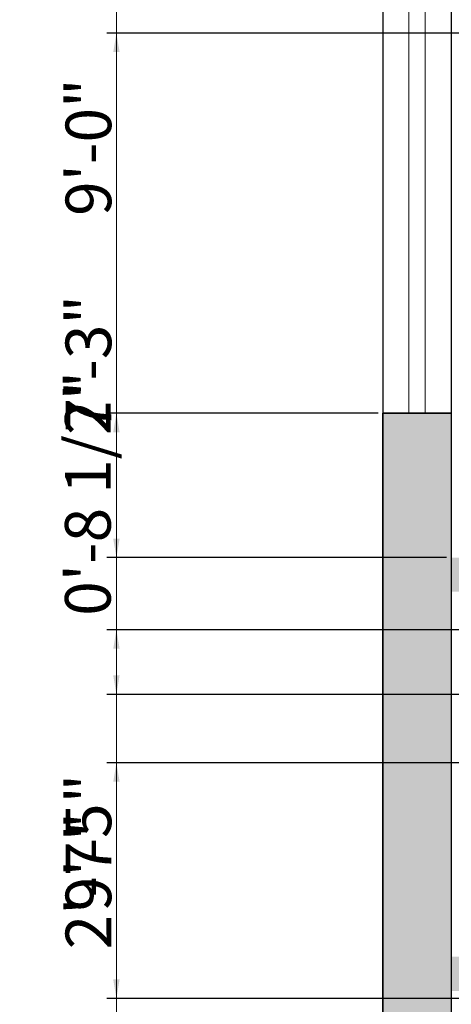
# Model space of a CAD drawing. Units: inches. Extents: x 2696 to 3240, y 1564 to 2310.
# Tile 14 of 76: x 2698 to 2755, y 1852 to 1982. Entities that reach past the tile are written whole.
import ezdxf

# ---------------------------------------------------------------- set-up
doc = ezdxf.new("R2010")
doc.units = ezdxf.units.IN
for name, color, linetype, lineweight in [('A-ANNO-DIMS', 3, 'Continuous', 18), ('A-WALL', 7, 'Continuous', 35), ('A-WALL-PATT', 9, 'Continuous', 13), ('WINDOW', 2, 'Continuous', 18)]:
    doc.layers.add(name, color=color, linetype=linetype, lineweight=lineweight)
doc.styles.add('TIMES NEW', font='times.ttf')
doc.dimstyles.new('Siddhuu', dxfattribs={"dimtxt": 6, "dimasz": 2.5, "dimexe": 1.25, "dimexo": 0.625, "dimtad": 1, "dimdec": 1, "dimlunit": 4, "dimtxsty": 'TIMES NEW', "dimcen": 2.5, "dimclrd": 256, "dimclre": 1, "dimclrt": 7, "dimadec": 0, "dimazin": 0, "dimtfac": 1, "dimtdec": 1, "dimtmove": 0, "dimatfit": 3, "dimfxl": 1, "dimtolj": 1, "dimlwd": -1, "dimarcsym": 0})

# ---------------------------------------------------------------- blocks, each defined once
blk = doc.blocks.new('WD_WIN4')
for p, q in [((-0.5, 0.5), (0.5, 0.5)), ((-0.5, 0.12), (0.5, 0.12)), ((-0.5, -0.12), (0.5, -0.12)), ((-0.5, -0.5), (0.5, -0.5))]:
    blk.add_line(p, q)
blk = doc.blocks.new('*D55')
at = {"layer": 'A-ANNO-DIMS', "color": 1, "lineweight": -2, "transparency": 16777216}
for p, q in [((3189.99, 1980.2), (2709.36, 1980.2)), ((3189.99, 1893.2), (2709.36, 1893.2))]:
    blk.add_line(p, q, dxfattribs=at)
at = {"layer": 'A-ANNO-DIMS', "transparency": 16777216}
blk.add_line((2710.61, 1895.7), (2710.61, 1977.7), dxfattribs=at)
for points in [[(2710.19, 1977.7), (2711.03, 1977.7), (2710.61, 1980.2)], [(2710.19, 1895.7), (2711.03, 1895.7), (2710.61, 1893.2)]]:
    blk.add_solid(points, dxfattribs=at)
at = {"layer": 'Defpoints', "color": 0, "transparency": 16777216}
for p in [(2710.61, 1980.2), (3190.61, 1980.2), (3190.61, 1893.2)]:
    blk.add_point(p, dxfattribs=at)
at = {"layer": 'A-ANNO-DIMS', "color": 7, "transparency": 16777216, "insert": (2706.93, 1936.7), "char_height": 6, "attachment_point": 5, "rotation": 90, "style": 'TIMES NEW'}
blk.add_mtext('\\A1;7\'-3"', dxfattribs=at)
blk = doc.blocks.new('*D57')
at = {"layer": 'A-ANNO-DIMS', "color": 1, "lineweight": -2, "transparency": 16777216}
for p, q in [((2754.61, 2018.58), (2754.61, 1568.95)), ((2956.71, 2018.58), (2956.71, 1568.95))]:
    blk.add_line(p, q, dxfattribs=at)
at = {"layer": 'A-ANNO-DIMS', "transparency": 16777216}
blk.add_line((2757.11, 1570.2), (2954.21, 1570.2), dxfattribs=at)
for points in [[(2757.11, 1570.62), (2757.11, 1569.78), (2754.61, 1570.2)], [(2954.21, 1570.62), (2954.21, 1569.78), (2956.71, 1570.2)]]:
    blk.add_solid(points, dxfattribs=at)
at = {"layer": 'Defpoints', "color": 0, "transparency": 16777216}
for p in [(2754.61, 2019.2), (2956.71, 2019.2), (2956.71, 1570.2)]:
    blk.add_point(p, dxfattribs=at)
at = {"layer": 'A-ANNO-DIMS', "color": 7, "transparency": 16777216, "insert": (2855.66, 1573.88), "char_height": 6, "attachment_point": 5, "style": 'TIMES NEW'}
blk.add_mtext('\\A1;16\'-10"', dxfattribs=at)
blk = doc.blocks.new('*D58')
at = {"layer": 'A-ANNO-DIMS', "color": 1, "lineweight": -2, "transparency": 16777216}
for p, q in [((2753.99, 2019.2), (2709.36, 2019.2)), ((2753.99, 1911.2), (2709.36, 1911.2))]:
    blk.add_line(p, q, dxfattribs=at)
at = {"layer": 'A-ANNO-DIMS', "transparency": 16777216}
blk.add_line((2710.61, 1913.7), (2710.61, 2016.7), dxfattribs=at)
for points in [[(2710.19, 2016.7), (2711.03, 2016.7), (2710.61, 2019.2)], [(2710.19, 1913.7), (2711.03, 1913.7), (2710.61, 1911.2)]]:
    blk.add_solid(points, dxfattribs=at)
at = {"layer": 'Defpoints', "color": 0, "transparency": 16777216}
for p in [(2710.61, 2019.2), (2754.61, 2019.2), (2754.61, 1911.2)]:
    blk.add_point(p, dxfattribs=at)
at = {"layer": 'A-ANNO-DIMS', "color": 7, "transparency": 16777216, "insert": (2706.93, 1965.2), "char_height": 6, "attachment_point": 5, "rotation": 90, "style": 'TIMES NEW'}
blk.add_mtext('\\A1;9\'-0"', dxfattribs=at)
blk = doc.blocks.new('*D68')
at = {"layer": 'A-ANNO-DIMS', "color": 1, "lineweight": -2, "transparency": 16777216}
for p, q in [((2745.61, 2261.58), (2745.61, 1568.95)), ((2782.83, 2261.58), (2782.83, 1568.95))]:
    blk.add_line(p, q, dxfattribs=at)
at = {"layer": 'A-ANNO-DIMS', "transparency": 16777216}
blk.add_line((2748.11, 1570.2), (2780.33, 1570.2), dxfattribs=at)
for points in [[(2748.11, 1570.62), (2748.11, 1569.78), (2745.61, 1570.2)], [(2780.33, 1570.62), (2780.33, 1569.78), (2782.83, 1570.2)]]:
    blk.add_solid(points, dxfattribs=at)
at = {"layer": 'Defpoints', "color": 0, "transparency": 16777216}
for p in [(2745.61, 2262.2), (2782.83, 2262.2), (2782.83, 1570.2)]:
    blk.add_point(p, dxfattribs=at)
at = {"layer": 'A-ANNO-DIMS', "color": 7, "transparency": 16777216, "insert": (2764.22, 1573.88), "char_height": 6, "attachment_point": 5, "style": 'TIMES NEW'}
blk.add_mtext('\\A1;3\'-1"', dxfattribs=at)
blk = doc.blocks.new('*D73')
at = {"layer": 'A-ANNO-DIMS', "color": 1, "lineweight": -2, "transparency": 16777216}
for p, q in [((2744.99, 1930.2), (2709.36, 1930.2)), ((2744.99, 1817.2), (2709.36, 1817.2))]:
    blk.add_line(p, q, dxfattribs=at)
at = {"layer": 'A-ANNO-DIMS', "transparency": 16777216}
blk.add_line((2710.61, 1927.7), (2710.61, 1819.7), dxfattribs=at)
for points in [[(2710.19, 1927.7), (2711.03, 1927.7), (2710.61, 1930.2)], [(2710.19, 1819.7), (2711.03, 1819.7), (2710.61, 1817.2)]]:
    blk.add_solid(points, dxfattribs=at)
at = {"layer": 'Defpoints', "color": 0, "transparency": 16777216}
for p in [(2745.61, 1930.2), (2710.61, 1817.2), (2745.61, 1817.2)]:
    blk.add_point(p, dxfattribs=at)
at = {"layer": 'A-ANNO-DIMS', "color": 7, "transparency": 16777216, "insert": (2706.93, 1873.7), "char_height": 6, "attachment_point": 5, "rotation": 90, "style": 'TIMES NEW'}
blk.add_mtext('\\A1;9\'-5"', dxfattribs=at)
blk = doc.blocks.new('*D78')
at = {"layer": 'A-ANNO-DIMS', "transparency": 16777216}
for p, q in [((2710.61, 1901.7), (2710.61, 1935.1)), ((2710.61, 1895.7), (2710.61, 1899.2))]:
    blk.add_line(p, q, dxfattribs=at)
at = {"layer": 'A-ANNO-DIMS', "color": 1, "lineweight": -2, "transparency": 16777216}
for p, q in [((3189.99, 1901.7), (2709.36, 1901.7)), ((3189.99, 1893.2), (2709.36, 1893.2))]:
    blk.add_line(p, q, dxfattribs=at)
at = {"layer": 'A-ANNO-DIMS', "transparency": 16777216}
for points in [[(2710.19, 1899.2), (2711.03, 1899.2), (2710.61, 1901.7)], [(2710.19, 1895.7), (2711.03, 1895.7), (2710.61, 1893.2)]]:
    blk.add_solid(points, dxfattribs=at)
at = {"layer": 'Defpoints', "color": 0, "transparency": 16777216}
for p in [(2710.61, 1901.7), (3190.61, 1901.7), (3190.61, 1893.2)]:
    blk.add_point(p, dxfattribs=at)
at = {"layer": 'A-ANNO-DIMS', "color": 7, "transparency": 16777216, "insert": (2706.85, 1919.65), "char_height": 6, "attachment_point": 5, "rotation": 90, "style": 'TIMES NEW'}
blk.add_mtext('\\A1;0\'-8 1/2"', dxfattribs=at)
blk = doc.blocks.new('*D79')
at = {"layer": 'A-ANNO-DIMS', "color": 1, "lineweight": -2, "transparency": 16777216}
for p, q in [((3189.99, 1884.2), (2709.36, 1884.2)), ((3189.99, 1853.2), (2709.36, 1853.2))]:
    blk.add_line(p, q, dxfattribs=at)
at = {"layer": 'A-ANNO-DIMS', "transparency": 16777216}
blk.add_line((2710.61, 1881.7), (2710.61, 1855.7), dxfattribs=at)
for points in [[(2710.19, 1881.7), (2711.03, 1881.7), (2710.61, 1884.2)], [(2710.19, 1855.7), (2711.03, 1855.7), (2710.61, 1853.2)]]:
    blk.add_solid(points, dxfattribs=at)
at = {"layer": 'Defpoints', "color": 0, "transparency": 16777216}
for p in [(3190.61, 1884.2), (2710.61, 1853.2), (3190.61, 1853.2)]:
    blk.add_point(p, dxfattribs=at)
at = {"layer": 'A-ANNO-DIMS', "color": 7, "transparency": 16777216, "insert": (2706.93, 1868.7), "char_height": 6, "attachment_point": 5, "rotation": 90, "style": 'TIMES NEW'}
blk.add_mtext('\\A1;2\'-7"', dxfattribs=at)

msp = doc.modelspace()

# ---------------------------------------------------------------- hatches: boundary and pattern name
at = {"layer": 'A-WALL-PATT', "transparency": 33554556}
h = msp.add_hatch(color=256, dxfattribs=at)
h.dxf.hatch_style = 1
h.paths.add_polyline_path([(2879.11, 2253.2), (2905.91, 2253.2), (2905.91, 2262.2), (2841.89, 2262.2), (2841.89, 2253.2), (2870.11, 2253.2), (2870.11, 2176.6), (2965.71, 2176.6), (2965.71, 2206.7), (2973.58, 2206.7), (2973.58, 2215.7), (2965.71, 2215.7), (2965.71, 2262.2), (2929.91, 2262.2), (2929.91, 2253.2), (2956.71, 2253.2), (2956.71, 2185.6), (2879.11, 2185.6)])
h.paths.add_polyline_path([(2782.83, 2262.2), (2745.61, 2262.2), (2745.61, 2228.73), (2754.61, 2228.73), (2754.61, 2253.2), (2782.83, 2253.2)])
h.paths.add_polyline_path([(2754.61, 2136.2), (2965.71, 2136.2), (2965.71, 2145.2), (2879.11, 2145.2), (2879.11, 2147.07), (2877.34, 2147.07), (2870.11, 2147.07), (2870.11, 2145.2), (2754.61, 2145.2), (2754.61, 2169.67), (2745.61, 2169.67), (2745.61, 2000.2), (2754.61, 2000.2), (2754.61, 2019.2), (2849.08, 2019.2), (2849.08, 2023.7), (2841.21, 2023.7), (2841.21, 2051.83), (2836.71, 2051.83), (2836.71, 2023.7), (2754.61, 2023.7), (2754.61, 2091.2), (2836.71, 2091.2), (2836.71, 2087.83), (2841.21, 2087.83), (2841.21, 2095.7), (2754.61, 2095.7)])
h.paths.add_polyline_path([(2965.71, 2136.2), (2956.71, 2136.2), (2956.71, 2023.7), (2885.08, 2023.7), (2885.08, 2019.2), (2956.71, 2019.2), (2956.71, 1950.58), (2965.71, 1950.58), (2965.71, 1980.2), (2973.58, 1980.2), (2973.58, 1989.2), (2965.71, 1989.2)])
h.paths.add_polyline_path([(2754.61, 1906.7), (2880.21, 1906.7), (2884.71, 1906.7), (2956.71, 1906.7), (2956.71, 1792.7), (2944.71, 1792.7), (2944.71, 1783.7), (2956.71, 1783.7), (2956.71, 1740.2), (2884.71, 1740.2), (2884.71, 1783.7), (2896.71, 1783.7), (2896.71, 1792.7), (2884.71, 1792.7), (2884.71, 1846.7), (2880.21, 1846.7), (2880.21, 1740.2), (2754.61, 1740.2), (2754.61, 1777.2), (2745.61, 1777.2), (2745.61, 1692.7), (2754.61, 1692.7), (2754.61, 1731.2), (2956.71, 1731.2), (2956.71, 1723.33), (2965.71, 1723.33), (2965.71, 1884.2), (2973.58, 1884.2), (2973.58, 1893.2), (2965.71, 1893.2), (2965.71, 1914.58), (2956.71, 1914.58), (2956.71, 1911.2), (2754.61, 1911.2), (2754.61, 1930.2), (2745.61, 1930.2), (2745.61, 1817.2), (2754.61, 1817.2), (2754.61, 1854.2), (2826.61, 1854.2), (2826.61, 1868.83), (2822.11, 1868.83), (2822.11, 1858.7), (2754.61, 1858.7)])
h.paths.add_polyline_path([(2965.71, 1656.2), (3008.24, 1656.2), (3008.24, 1665.2), (2965.71, 1665.2), (2965.71, 1693.33), (2956.71, 1693.33), (2956.71, 1686.2), (2934.58, 1686.2), (2934.58, 1681.7), (2956.71, 1681.7), (2956.71, 1614.2), (2896.71, 1614.2), (2896.71, 1681.7), (2904.58, 1681.7), (2904.58, 1686.2), (2892.21, 1686.2), (2892.21, 1614.2), (2858.41, 1614.2), (2858.41, 1605.2), (2965.71, 1605.2)])
h.paths.add_polyline_path([(2788.41, 1614.2), (2754.61, 1614.2), (2754.61, 1652.7), (2745.61, 1652.7), (2745.61, 1605.2), (2788.41, 1605.2)])
h.paths.add_polyline_path([(3199.61, 1633.05), (3190.61, 1633.05), (3190.61, 1614.2), (3082.61, 1614.2), (3082.61, 1665.2), (3070.24, 1665.2), (3070.24, 1656.2), (3078.11, 1656.2), (3078.11, 1605.2), (3199.61, 1605.2)])
h.paths.add_polyline_path([(3199.61, 1702.05), (3190.61, 1702.05), (3190.61, 1699.7), (3106.61, 1699.7), (3106.61, 1747.7), (3190.61, 1747.7), (3190.61, 1752.2), (3082.61, 1752.2), (3082.61, 1760.08), (3078.11, 1760.08), (3078.11, 1747.7), (3102.11, 1747.7), (3102.11, 1699.7), (3078.11, 1699.7), (3078.11, 1695.2), (3190.61, 1695.2), (3190.61, 1676.35), (3199.61, 1676.35)])
h.paths.add_polyline_path([(3199.61, 1783.2), (3190.61, 1783.2), (3190.61, 1745.35), (3199.61, 1745.35)])
h.paths.add_polyline_path([(3082.61, 1884.2), (3190.61, 1884.2), (3190.61, 1853.2), (3199.61, 1853.2), (3199.61, 1901.7), (3190.61, 1901.7), (3190.61, 1893.2), (3005.58, 1893.2), (3005.58, 1891.28), (3005.58, 1884.2), (3078.11, 1884.2), (3078.11, 1792.08), (3082.61, 1792.08)])
h.paths.add_polyline_path([(3199.61, 1994.7), (3190.61, 1994.7), (3190.61, 1989.2), (3073.71, 1989.2), (3073.71, 2034.2), (3069.21, 2034.2), (3069.21, 1989.2), (3005.58, 1989.2), (3005.58, 1980.2), (3190.61, 1980.2), (3190.61, 1971.7), (3199.61, 1971.7)])
h.paths.add_polyline_path([(3199.61, 2155.2), (3190.61, 2155.2), (3190.61, 2064.7), (3199.61, 2064.7)])
h.paths.add_polyline_path([(3190.61, 2074.7), (3106.61, 2074.7), (3106.61, 2122.7), (3190.61, 2122.7), (3190.61, 2127.2), (3082.71, 2127.2), (3082.71, 2135.08), (3073.71, 2135.08), (3073.71, 2122.7), (3102.11, 2122.7), (3102.11, 2074.7), (3069.21, 2074.7), (3069.21, 2070.2), (3190.61, 2070.2)])
h.paths.add_polyline_path([(3082.71, 2253.2), (3190.61, 2253.2), (3190.61, 2225.2), (3199.61, 2225.2), (3199.61, 2262.2), (3073.71, 2262.2), (3073.71, 2215.7), (3035.58, 2215.7), (3035.58, 2206.7), (3073.71, 2206.7), (3073.71, 2171.08), (3082.71, 2171.08)])

# ---------------------------------------------------------------- linework, layer by layer
at = {"layer": 'A-WALL'}
for p in [(2745.61, 1817.2), (2754.61, 1930.2)]:
    msp.add_line(p, (2745.61, 1930.2), dxfattribs=at)

# ---------------------------------------------------------------- block references
at = {"layer": 'WINDOW', "xscale": 70, "yscale": 8.999999999999545, "zscale": 70, "rotation": 270}
msp.add_blockref('WD_WIN4', (2750.11, 1965.2), dxfattribs=at)

# ---------------------------------------------------------------- dimensions: what is measured, and where the dimension line sits
at = {"layer": 'A-ANNO-DIMS'}
for base, p1, p2, picture, middle in [((2782.83, 1570.2), (2745.61, 2262.2), (2782.83, 2262.2), '*D68', (2764.22, 1573.88)), ((2956.71, 1570.2), (2754.61, 2019.2), (2956.71, 2019.2), '*D57', (2855.66, 1573.88))]:
    dim = msp.add_linear_dim(base=base, p1=p1, p2=p2, dimstyle='Siddhuu', override={"dimdec": 1, "dimlfac": 1, "dimrnd": 0, "dimzin": 1, "dimdsep": 46, "dimlunit": 4, "dimfrac": 2}, dxfattribs=at)
    dim.commit()
    dim.dimension.update_dxf_attribs({"geometry": picture, "text_midpoint": middle})
for base, p1, p2, picture, middle in [((2710.61, 2019.2), (2754.61, 1911.2), (2754.61, 2019.2), '*D58', (2706.93, 1965.2)), ((2710.61, 1980.2), (3190.61, 1893.2), (3190.61, 1980.2), '*D55', (2706.93, 1936.7)), ((2710.61, 1901.7), (3190.61, 1893.2), (3190.61, 1901.7), '*D78', (2706.85, 1919.65)), ((2710.61, 1817.2), (2745.61, 1930.2), (2745.61, 1817.2), '*D73', (2706.93, 1873.7)), ((2710.61, 1853.2), (3190.61, 1884.2), (3190.61, 1853.2), '*D79', (2706.93, 1868.7))]:
    dim = msp.add_linear_dim(base=base, p1=p1, p2=p2, angle=90, dimstyle='Siddhuu', override={"dimdec": 1, "dimlfac": 1, "dimrnd": 0, "dimzin": 1, "dimdsep": 46, "dimlunit": 4, "dimfrac": 2}, dxfattribs=at)
    dim.commit()
    dim.dimension.update_dxf_attribs({"geometry": picture, "text_midpoint": middle})

doc.saveas('drawing.dxf')
